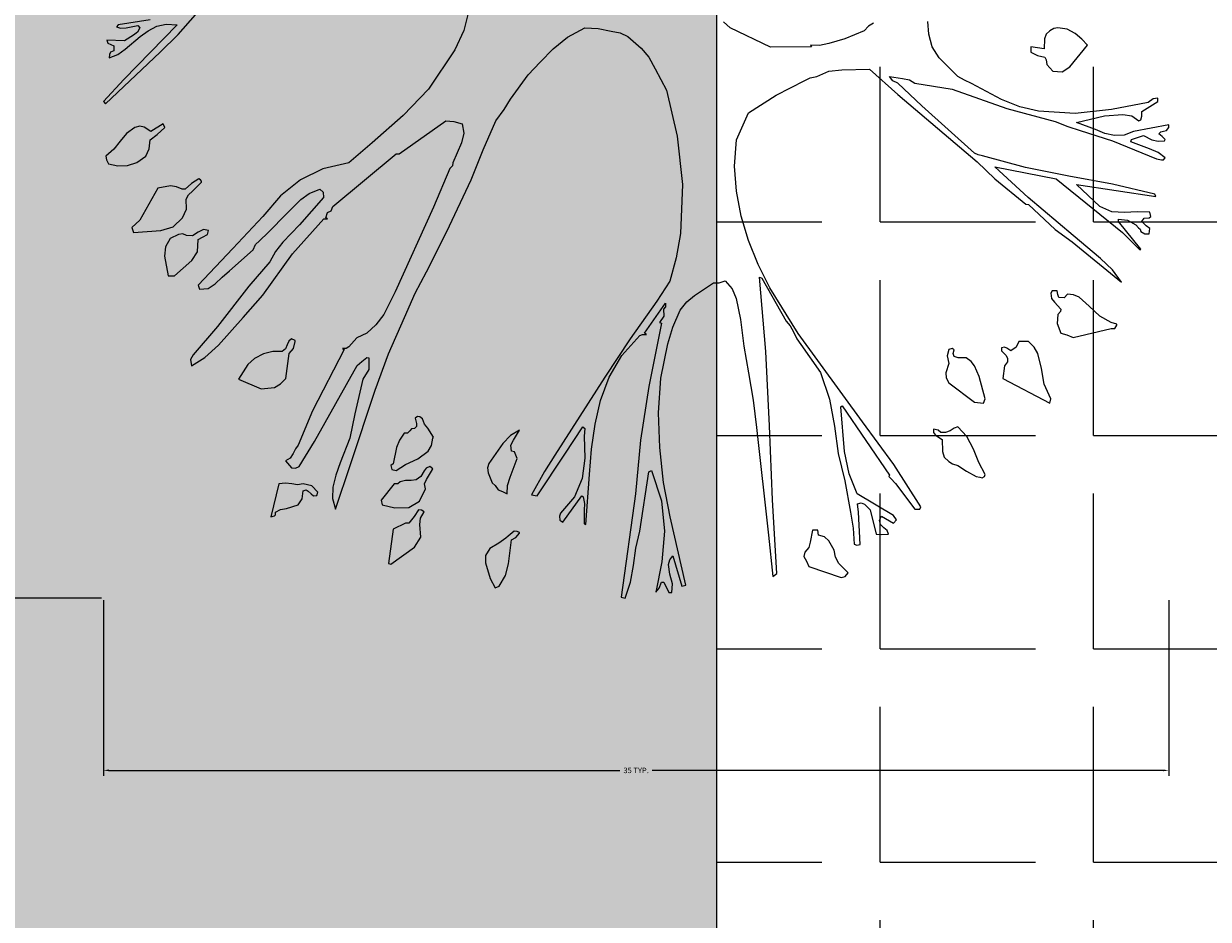
# Model space of a CAD drawing. Units: inches. Extents: x 84 to 1044, y -280 to 906.
# Tile 11 of 105: x 482 to 521, y -79 to -49. Entities that reach past the tile are written whole.
import ezdxf

# ---------------------------------------------------------------- set-up
doc = ezdxf.new("R2010")
doc.units = ezdxf.units.IN
for name, color, linetype, lineweight in [('A-ANNO-DIMS', 2, 'Continuous', 18), ('L-HRDS', 32, 'Continuous', 18), ('L-PLNT', 114, 'Continuous', 15)]:
    doc.layers.add(name, color=color, linetype=linetype, lineweight=lineweight)
doc.layers.add('L-HRDS-PATT', color=23, linetype='Continuous', lineweight=9, true_color=0xc2877b)
doc.layers.add('L-PLNT-PATT', color=9, linetype='Continuous', lineweight=9, true_color=0xafd9aa)
doc.styles.get("Standard").update_dxf_attribs({"font": 'arial.ttf'})
doc.dimstyles.get("Standard").update_dxf_attribs({"dimtxt": 0.18, "dimasz": 0.18, "dimexe": 0.18, "dimexo": 0.0625, "dimgap": 0.09, "dimtad": 0, "dimtih": 1, "dimtoh": 1, "dimdec": 4, "dimzin": 0, "dimdsep": 46, "dimtxsty": 'Standard', "dimcen": 0.09, "dimadec": 0, "dimazin": 0, "dimtfac": 1, "dimtdec": 4, "dimtofl": 0, "dimtmove": 0, "dimatfit": 3, "dimfxl": 1, "dimtolj": 1, "dimtzin": 0, "dimarcsym": 0})

# ---------------------------------------------------------------- blocks, each defined once
blk = doc.blocks.new('A$C37E508DF')
for p, q in [((0.9287, 0.7825), (0.936, 0.7542)), ((1.3151, 0.7487), (1.2919, 0.7752)), ((0.1244, 0.7504), (0.1351, 0.7559)), ((0.1351, 0.7559), (0.1471, 0.7577)), ((0.1471, 0.7577), (0.1527, 0.7568)), ((0.1527, 0.7568), (0.1578, 0.7538)), ((0.3186, 0.7491), (0.3199, 0.7662)), ((0.3919, 0.7641), (0.3988, 0.7598)), ((0.3988, 0.7598), (0.4043, 0.7538)), ((0.5287, 0.7319), (0.5823, 0.7577)), ((0.5823, 0.7577), (0.5913, 0.7658)), ((0.7577, 0.7568), (0.7401, 0.7534)), ((0.7752, 0.7577), (0.7577, 0.7568)), ((0.798, 0.7452), (0.7752, 0.7577)), ((1.3309, 0.7624), (1.3164, 0.7615)), ((1.3164, 0.7615), (1.3871, 0.6891)), ((1.3434, 0.7598), (1.3309, 0.7624)), ((1.355, 0.7538), (1.3434, 0.7598)), ((1.352, 0.7684), (1.3948, 0.7615)), ((1.3687, 0.7607), (1.3657, 0.7577)), ((1.3657, 0.7577), (1.3691, 0.7521)), ((1.3841, 0.7577), (1.3687, 0.7607)), ((1.3914, 0.7572), (1.3841, 0.7577)), ((1.397, 0.759), (1.3914, 0.7572)), ((1.3948, 0.7615), (1.397, 0.759)), ((0.1081, 0.7349), (0.1153, 0.7427)), ((0.1153, 0.7427), (0.1244, 0.7504)), ((0.1578, 0.7538), (0.1629, 0.7491)), ((0.1629, 0.7491), (0.1651, 0.7431)), ((0.1651, 0.7431), (0.1655, 0.7298)), ((0.3139, 0.7324), (0.3186, 0.7491)), ((0.4043, 0.7538), (0.4301, 0.7431)), ((0.4301, 0.7431), (0.4515, 0.7371)), ((0.7182, 0.7461), (0.7002, 0.7307)), ((0.7285, 0.7512), (0.7182, 0.7461)), ((0.7401, 0.7534), (0.7285, 0.7512)), ((0.8173, 0.7298), (0.798, 0.7452)), ((0.936, 0.7542), (0.9476, 0.7285)), ((1.3391, 0.7255), (1.3151, 0.7487)), ((1.3653, 0.7461), (1.355, 0.7538)), ((1.3854, 0.7294), (1.3653, 0.7461)), ((1.3691, 0.7521), (1.3743, 0.7482)), ((1.3743, 0.7482), (1.3863, 0.7405)), ((1.3863, 0.7405), (1.4099, 0.7414)), ((1.4099, 0.7414), (1.4086, 0.7375)), ((0.1312, 0.7058), (0.1081, 0.7349)), ((0.1655, 0.7298), (0.1831, 0.7324)), ((0.1831, 0.7255), (0.1741, 0.7208)), ((0.1831, 0.7324), (0.1831, 0.7255)), ((0.3049, 0.7178), (0.3139, 0.7324)), ((0.4515, 0.7371), (0.4635, 0.7341)), ((0.4635, 0.7341), (0.4755, 0.7349)), ((0.4755, 0.7349), (0.4742, 0.7324)), ((0.4742, 0.7324), (0.5287, 0.7319)), ((0.7002, 0.7307), (0.6903, 0.7186)), ((0.8344, 0.7122), (0.8173, 0.7298)), ((0.9476, 0.7285), (0.9828, 0.6762)), ((1.4116, 0.6569), (1.3391, 0.7255)), ((1.3953, 0.7221), (1.3854, 0.7294)), ((1.4086, 0.7375), (1.4004, 0.7337)), ((1.4004, 0.7337), (1.4004, 0.7272)), ((1.4004, 0.7272), (1.4047, 0.7255)), ((1.4047, 0.7255), (1.406, 0.7221)), ((0.1621, 0.7092), (0.1539, 0.7002)), ((0.1629, 0.7152), (0.1621, 0.7092)), ((0.1646, 0.7186), (0.1629, 0.7152)), ((0.1741, 0.7208), (0.1646, 0.7186)), ((0.28, 0.6933), (0.3049, 0.7178)), ((0.6903, 0.7186), (0.6818, 0.7032)), ((0.8503, 0.6951), (0.8344, 0.7122)), ((1.4064, 0.7178), (1.3953, 0.7221)), ((1.406, 0.7221), (1.4064, 0.7178)), ((0.1415, 0.6994), (0.1312, 0.7058)), ((0.1539, 0.7002), (0.1415, 0.6994)), ((0.271, 0.6882), (0.28, 0.6933)), ((0.3709, 0.6933), (0.3533, 0.6903)), ((0.3975, 0.7028), (0.3598, 0.6693)), ((0.3662, 0.6873), (0.3709, 0.6933)), ((0.4339, 0.7019), (0.3975, 0.7028)), ((0.4515, 0.7002), (0.4339, 0.7019)), ((0.4674, 0.6933), (0.4515, 0.7002)), ((0.476, 0.6912), (0.4674, 0.6933)), ((0.6818, 0.7032), (0.6667, 0.6749)), ((0.8739, 0.6629), (0.8503, 0.6951)), ((0.2877, 0.6762), (0.2152, 0.6505)), ((0.2221, 0.6625), (0.262, 0.6839)), ((0.262, 0.6839), (0.271, 0.6882)), ((0.337, 0.6843), (0.2877, 0.6762)), ((0.328, 0.6543), (0.3598, 0.6843)), ((0.3443, 0.6886), (0.337, 0.6843)), ((0.3533, 0.6903), (0.3443, 0.6886)), ((0.3598, 0.6843), (0.3662, 0.6873)), ((0.4832, 0.6878), (0.476, 0.6912)), ((0.521, 0.6685), (0.4832, 0.6878)), ((0.9828, 0.6762), (1.0162, 0.6415)), ((1.3871, 0.6891), (1.4141, 0.6599)), ((0.0146, 0.6599), (0.0146, 0.6642)), ((0.0146, 0.6642), (0.0206, 0.6633)), ((0.0206, 0.6633), (0.0274, 0.6586)), ((0.1977, 0.6526), (0.2221, 0.6625)), ((0.3598, 0.6693), (0.2543, 0.5797)), ((0.5578, 0.6449), (0.521, 0.6685)), ((0.6667, 0.6749), (0.6526, 0.614)), ((0.8824, 0.6492), (0.8739, 0.6629)), ((0.036, 0.6466), (0.0146, 0.6599)), ((0.0274, 0.6586), (0.0759, 0.6492)), ((0.0356, 0.6406), (0.036, 0.6466)), ((0.0759, 0.6492), (0.1244, 0.644)), ((0.1244, 0.644), (0.1728, 0.647)), ((0.2152, 0.6505), (0.1509, 0.6333)), ((0.1728, 0.647), (0.1977, 0.6526)), ((0.2581, 0.5913), (0.328, 0.6543)), ((0.5737, 0.6089), (0.5578, 0.6449)), ((0.8932, 0.6342), (0.8824, 0.6492)), ((1.4141, 0.6599), (1.4116, 0.6569)), ((0, 0.629), (0.0467, 0.62)), ((0, 0.6252), (0, 0.629)), ((0.0369, 0.6355), (0.0356, 0.6406)), ((0.0399, 0.6342), (0.0369, 0.6355)), ((0.0489, 0.641), (0.0399, 0.6342)), ((0.0609, 0.6428), (0.0489, 0.641)), ((0.0853, 0.641), (0.0609, 0.6428)), ((0.1226, 0.632), (0.0853, 0.641)), ((0.0973, 0.6226), (0.1226, 0.632)), ((0.1509, 0.6333), (0.1342, 0.6265)), ((0.9103, 0.5956), (0.8932, 0.6342)), ((0.9382, 0.6303), (0.936, 0.6179)), ((0.9493, 0.6333), (0.9382, 0.6303)), ((0.9596, 0.6342), (0.9493, 0.6333)), ((1.0218, 0.5904), (0.9596, 0.6342)), ((1.0162, 0.6415), (1.0574, 0.605)), ((1.3327, 0.6252), (1.3348, 0.6303)), ((1.3348, 0.6303), (1.3511, 0.62)), ((0.003, 0.6213), (0, 0.6252)), ((0.0069, 0.6204), (0.003, 0.6213)), ((0.0107, 0.6196), (0.0069, 0.6204)), ((0.0086, 0.6132), (0.0133, 0.617)), ((0.0133, 0.617), (0.0107, 0.6196)), ((0.0334, 0.6145), (0.0223, 0.6089)), ((0.0416, 0.6119), (0.0334, 0.6145)), ((0.0467, 0.62), (0.0592, 0.6153)), ((0.0592, 0.6153), (0.072, 0.6149)), ((0.072, 0.6149), (0.0849, 0.6175)), ((0.1175, 0.6213), (0.0746, 0.6076)), ((0.0849, 0.6175), (0.0973, 0.6226)), ((0.1342, 0.6265), (0.1175, 0.6213)), ((0.6526, 0.614), (0.6457, 0.5497)), ((0.936, 0.6179), (0.939, 0.605)), ((1.343, 0.6162), (1.3327, 0.6252)), ((1.352, 0.6089), (1.343, 0.6162)), ((1.3511, 0.62), (1.3601, 0.6256)), ((1.3601, 0.6256), (1.3661, 0.6269)), ((1.3661, 0.6269), (1.3725, 0.6252)), ((1.3725, 0.6252), (1.3837, 0.6175)), ((1.3837, 0.6175), (1.3918, 0.6072)), ((0.0047, 0.6093), (0.0086, 0.6132)), ((0.0056, 0.6076), (0.0047, 0.6093)), ((0.0141, 0.6072), (0.0056, 0.6076)), ((0.0223, 0.6089), (0.0141, 0.6072)), ((0.0746, 0.6076), (0.0163, 0.5836)), ((0.0257, 0.5969), (0.0506, 0.6063)), ((0.0493, 0.6093), (0.0416, 0.6119)), ((0.0506, 0.6063), (0.0493, 0.6093)), ((0.5763, 0.5741), (0.5737, 0.6089)), ((0.939, 0.605), (0.9506, 0.5784)), ((1.0574, 0.605), (1.0883, 0.5784)), ((1.3533, 0.5969), (1.352, 0.6089)), ((1.3918, 0.6072), (1.4004, 0.5964)), ((0.0047, 0.5849), (0.0141, 0.5921)), ((0.0069, 0.5823), (0.0047, 0.5849)), ((0.0099, 0.5823), (0.0069, 0.5823)), ((0.0163, 0.5836), (0.0099, 0.5823)), ((0.0141, 0.5921), (0.0257, 0.5969)), ((0.1904, 0.5724), (0.2474, 0.5879)), ((0.2474, 0.5879), (0.253, 0.5892)), ((0.253, 0.5892), (0.2581, 0.5913)), ((0.9262, 0.5557), (0.9103, 0.5956)), ((1.0256, 0.5904), (1.0218, 0.5904)), ((1.1097, 0.5205), (1.0256, 0.5904)), ((1.358, 0.5874), (1.3533, 0.5969)), ((1.37, 0.5789), (1.358, 0.5874)), ((1.4004, 0.5964), (1.4111, 0.5874)), ((1.4103, 0.5823), (1.4077, 0.5771)), ((1.4111, 0.5874), (1.4103, 0.5823)), ((0.1325, 0.5608), (0.1904, 0.5724)), ((0.2311, 0.5729), (0.1496, 0.557)), ((0.1869, 0.5325), (0.2311, 0.5729)), ((0.2543, 0.5797), (0.2311, 0.557)), ((0.5737, 0.5407), (0.5763, 0.5741)), ((0.9506, 0.5784), (0.951, 0.5746)), ((0.951, 0.5746), (0.9545, 0.5711)), ((0.9545, 0.5711), (0.9759, 0.5193)), ((1.0883, 0.5784), (1.123, 0.5703)), ((1.123, 0.5703), (1.1526, 0.5557)), ((1.3824, 0.575), (1.37, 0.5789)), ((1.3953, 0.5746), (1.3824, 0.575)), ((1.4077, 0.5771), (1.3953, 0.5746)), ((0.1496, 0.557), (0.0613, 0.4858)), ((0.0746, 0.5501), (0.1325, 0.5608)), ((0.2311, 0.557), (0.1899, 0.5235)), ((0.9583, 0.4871), (0.9262, 0.5557)), ((1.1526, 0.5557), (1.1792, 0.5347)), ((1.2842, 0.554), (1.2855, 0.5557)), ((1.2842, 0.5527), (1.2842, 0.554)), ((1.2958, 0.5407), (1.2842, 0.5527)), ((1.2855, 0.5557), (1.2876, 0.557)), ((1.2876, 0.557), (1.2971, 0.551)), ((1.2971, 0.551), (1.3057, 0.5433)), ((0.1226, 0.5497), (0.0171, 0.5338)), ((0.0171, 0.5338), (0.0184, 0.5368)), ((0.0184, 0.5368), (0.0746, 0.5501)), ((0.0917, 0.5205), (0.1226, 0.5497)), ((0.5677, 0.5077), (0.5737, 0.5407)), ((0.6457, 0.5497), (0.6483, 0.4845)), ((1.1226, 0.5394), (1.1221, 0.5325)), ((1.1268, 0.5433), (1.1226, 0.5394)), ((1.141, 0.5377), (1.1268, 0.5433)), ((1.1521, 0.5296), (1.141, 0.5377)), ((1.1792, 0.5347), (1.2027, 0.5072)), ((1.3014, 0.536), (1.2958, 0.5407)), ((1.3044, 0.53), (1.3014, 0.536)), ((1.3057, 0.5433), (1.3099, 0.5433)), ((1.3099, 0.5433), (1.3172, 0.5467)), ((1.3172, 0.5467), (1.3254, 0.548)), ((1.3254, 0.548), (1.3421, 0.5446)), ((1.3421, 0.5446), (1.3657, 0.5021)), ((0.0755, 0.5133), (0.0917, 0.5205)), ((0.1269, 0.482), (0.1869, 0.5325)), ((0.1861, 0.5231), (0.1509, 0.4897)), ((0.1899, 0.5235), (0.1861, 0.5231)), ((0.9759, 0.5193), (1.0269, 0.4069)), ((1.1118, 0.5145), (1.1097, 0.5205)), ((1.1221, 0.5325), (1.1539, 0.4961)), ((1.1706, 0.5111), (1.1521, 0.5296)), ((1.3039, 0.5167), (1.3044, 0.53)), ((0.024, 0.5072), (0.0253, 0.5128)), ((0.0262, 0.5055), (0.024, 0.5072)), ((0.0253, 0.5128), (0.042, 0.5133)), ((0.0326, 0.5047), (0.0262, 0.5055)), ((0.036, 0.5004), (0.0326, 0.5047)), ((0.042, 0.5133), (0.0587, 0.5124)), ((0.0669, 0.5034), (0.0549, 0.5021)), ((0.0587, 0.5124), (0.0755, 0.5133)), ((0.0669, 0.5004), (0.0669, 0.5034)), ((0.5578, 0.4751), (0.5677, 0.5077)), ((1.117, 0.5124), (1.1118, 0.5145)), ((1.1191, 0.5055), (1.117, 0.5124)), ((1.117, 0.5042), (1.1191, 0.5055)), ((1.1217, 0.5042), (1.117, 0.5042)), ((1.1633, 0.4575), (1.1217, 0.5042)), ((1.1955, 0.4858), (1.1706, 0.5111)), ((1.2027, 0.5072), (1.2426, 0.4644)), ((1.3091, 0.5055), (1.3039, 0.5167)), ((1.3215, 0.4935), (1.3091, 0.5055)), ((0.0253, 0.491), (0.03, 0.4948)), ((0.0262, 0.4841), (0.0253, 0.491)), ((0.03, 0.4948), (0.036, 0.5004)), ((0.0369, 0.4639), (0.0669, 0.5004)), ((0.0382, 0.4905), (0.0369, 0.4871)), ((0.0403, 0.4922), (0.0382, 0.4905)), ((0.0437, 0.4961), (0.0403, 0.4922)), ((0.0549, 0.5021), (0.0437, 0.4961)), ((0.1509, 0.4897), (0.1282, 0.4734)), ((1.1539, 0.4961), (1.1762, 0.4729)), ((1.2748, 0.4884), (1.2812, 0.4897)), ((1.2761, 0.4832), (1.2748, 0.4884)), ((1.2812, 0.4897), (1.2885, 0.4862)), ((1.3382, 0.4884), (1.3215, 0.4935)), ((1.3743, 0.4858), (1.3382, 0.4884)), ((1.3657, 0.5021), (1.3764, 0.4927)), ((1.3764, 0.4927), (1.3743, 0.4858)), ((0.0317, 0.4841), (0.0262, 0.4841)), ((0.0369, 0.4871), (0.0317, 0.4841)), ((0.0613, 0.4858), (0.0386, 0.4627)), ((0.1282, 0.4734), (0.0626, 0.4198)), ((0.0905, 0.4515), (0.1269, 0.482)), ((0.545, 0.4434), (0.5578, 0.4751)), ((0.6483, 0.4845), (0.6539, 0.4524)), ((0.9853, 0.4335), (0.9583, 0.4871)), ((1.1762, 0.4729), (1.1856, 0.4605)), ((1.207, 0.4747), (1.1955, 0.4858)), ((1.2122, 0.47), (1.207, 0.4747)), ((1.2825, 0.4798), (1.2761, 0.4832)), ((1.2885, 0.4764), (1.2825, 0.4798)), ((1.2885, 0.4862), (1.2962, 0.4815)), ((1.2894, 0.4601), (1.2885, 0.4764)), ((1.2962, 0.4815), (1.3039, 0.482)), ((1.3039, 0.482), (1.3087, 0.4841)), ((1.3087, 0.4841), (1.3147, 0.4832)), ((1.3147, 0.4832), (1.3258, 0.4777)), ((1.3258, 0.4777), (1.3318, 0.4669)), ((0.0386, 0.4627), (0.0369, 0.4639)), ((1.2027, 0.4026), (1.1633, 0.4575)), ((1.1856, 0.4605), (1.1933, 0.4468)), ((1.2156, 0.4627), (1.2122, 0.47)), ((1.2469, 0.4348), (1.2156, 0.4627)), ((1.2426, 0.4644), (1.2885, 0.4159)), ((1.2967, 0.4485), (1.2894, 0.4601)), ((1.3318, 0.4669), (1.3331, 0.4545)), ((0.0746, 0.4361), (0.0905, 0.4515)), ((0.5295, 0.4125), (0.545, 0.4434)), ((0.6539, 0.4524), (0.6625, 0.4211)), ((1.1933, 0.4468), (1.2212, 0.4146)), ((1.3082, 0.4386), (1.2967, 0.4485)), ((1.3331, 0.4545), (1.3284, 0.4284)), ((0.0626, 0.4198), (0.0746, 0.4361)), ((0.5403, 0.4254), (0.5081, 0.3679)), ((0.5347, 0.3276), (0.5433, 0.4266)), ((0.5433, 0.4266), (0.5403, 0.4254)), ((1.0003, 0.4052), (0.9853, 0.4335)), ((1.2568, 0.4266), (1.2469, 0.4348)), ((1.2658, 0.4176), (1.2568, 0.4266)), ((1.3198, 0.4284), (1.3082, 0.4386)), ((1.3284, 0.4284), (1.3198, 0.4284)), ((0.4922, 0.3516), (0.5295, 0.4125)), ((0.5797, 0.4112), (0.5741, 0.3983)), ((0.5887, 0.4215), (0.5797, 0.4112)), ((0.5969, 0.4189), (0.5887, 0.4215)), ((0.6046, 0.4189), (0.5969, 0.4189)), ((0.6295, 0.4022), (0.6046, 0.4189)), ((0.6625, 0.4211), (0.6796, 0.3945)), ((1.2212, 0.4146), (1.2628, 0.361)), ((1.2752, 0.4116), (1.2658, 0.4176)), ((1.2868, 0.4108), (1.2752, 0.4116)), ((1.2885, 0.4159), (1.2868, 0.4108)), ((0.1055, 0.388), (0.1192, 0.4001)), ((0.1192, 0.4001), (0.1265, 0.4031)), ((0.1265, 0.4031), (0.1346, 0.4039)), ((0.1346, 0.4039), (0.1389, 0.3992)), ((0.1389, 0.3992), (0.1458, 0.3996)), ((0.1518, 0.3932), (0.1432, 0.3842)), ((0.1458, 0.3996), (0.1471, 0.4035)), ((0.1471, 0.4035), (0.1484, 0.4082)), ((0.1484, 0.4082), (0.1548, 0.4082)), ((0.1556, 0.3983), (0.1518, 0.3932)), ((0.1548, 0.4082), (0.1565, 0.4052)), ((0.1565, 0.4052), (0.1556, 0.3983)), ((0.5741, 0.3983), (0.5686, 0.3705)), ((0.6397, 0.3936), (0.6295, 0.4022)), ((0.6487, 0.3825), (0.6397, 0.3936)), ((0.6796, 0.3945), (0.7148, 0.3447)), ((1.0145, 0.373), (1.0003, 0.4052)), ((1.0269, 0.4069), (1.0419, 0.3769)), ((1.2289, 0.373), (1.2027, 0.4026)), ((0.0917, 0.3748), (0.1055, 0.388)), ((0.1432, 0.3842), (0.1436, 0.3808)), ((0.1436, 0.3808), (0.1471, 0.3769)), ((0.6582, 0.3602), (0.6487, 0.3825)), ((0.6959, 0.352), (0.668, 0.3919)), ((0.668, 0.3919), (0.668, 0.3872)), ((0.668, 0.3872), (0.6706, 0.3842)), ((0.6706, 0.3842), (0.6702, 0.3748)), ((0.069, 0.364), (0.0763, 0.3662)), ((0.069, 0.3627), (0.069, 0.364)), ((0.0716, 0.3585), (0.069, 0.3627)), ((0.0763, 0.3662), (0.0917, 0.3748)), ((0.1484, 0.3649), (0.1432, 0.352)), ((0.1471, 0.3769), (0.1484, 0.3649)), ((0.5025, 0.3619), (0.4982, 0.3537)), ((0.5081, 0.3679), (0.5025, 0.3619)), ((0.5686, 0.3705), (0.5643, 0.3349)), ((0.6702, 0.3748), (0.6762, 0.3662)), ((0.6762, 0.3662), (0.6732, 0.3653)), ((0.6732, 0.3653), (0.6903, 0.2813)), ((1.0359, 0.3246), (1.0145, 0.373)), ((1.0419, 0.3769), (1.0527, 0.3632)), ((1.0527, 0.3632), (1.0647, 0.352)), ((1.2615, 0.3362), (1.2289, 0.373)), ((0.0763, 0.3585), (0.0716, 0.3585)), ((0.1269, 0.3464), (0.0763, 0.3585)), ((0.1355, 0.3499), (0.1269, 0.3464)), ((0.1432, 0.352), (0.1355, 0.3499)), ((0.4065, 0.2345), (0.4922, 0.3516)), ((0.4982, 0.3537), (0.4939, 0.3447)), ((0.665, 0.3379), (0.6582, 0.3602)), ((0.6933, 0.3503), (0.6959, 0.352)), ((0.6985, 0.3503), (0.6933, 0.3503)), ((0.7023, 0.349), (0.6985, 0.3503)), ((0.7259, 0.3224), (0.7023, 0.349)), ((1.0647, 0.352), (1.078, 0.346)), ((1.078, 0.346), (1.0883, 0.334)), ((1.2628, 0.361), (1.2949, 0.3233)), ((0.1737, 0.325), (0.1788, 0.3336)), ((0.1788, 0.3336), (0.1861, 0.3409)), ((0.1861, 0.3409), (0.199, 0.3409)), ((0.199, 0.3409), (0.2024, 0.3336)), ((0.2024, 0.3336), (0.2097, 0.3289)), ((0.2097, 0.3289), (0.2148, 0.3323)), ((0.2148, 0.3323), (0.2182, 0.3336)), ((0.2182, 0.3336), (0.2221, 0.3327)), ((0.2221, 0.3327), (0.2221, 0.3289)), ((0.2851, 0.3302), (0.2877, 0.3319)), ((0.2877, 0.3319), (0.292, 0.3306)), ((0.292, 0.3306), (0.2941, 0.322)), ((0.4884, 0.337), (0.4622, 0.2997)), ((0.4939, 0.3447), (0.4884, 0.337)), ((0.5643, 0.3349), (0.5578, 0.2993)), ((0.6745, 0.2924), (0.665, 0.3379)), ((0.7148, 0.3447), (0.7487, 0.2937)), ((1.0883, 0.334), (1.0921, 0.3319)), ((1.0921, 0.3319), (1.0968, 0.3319)), ((1.0968, 0.3319), (1.0947, 0.3306)), ((1.0947, 0.3306), (1.1367, 0.2491)), ((1.1599, 0.3426), (1.1646, 0.3447)), ((1.1599, 0.3413), (1.1599, 0.3426)), ((1.162, 0.3319), (1.1599, 0.3413)), ((1.1676, 0.325), (1.162, 0.3319)), ((1.1646, 0.3447), (1.168, 0.3417)), ((1.168, 0.3417), (1.1702, 0.3366)), ((1.1702, 0.3366), (1.1727, 0.3314)), ((1.1727, 0.3314), (1.177, 0.3276)), ((1.2795, 0.3199), (1.2615, 0.3362)), ((0.1689, 0.3053), (0.1737, 0.325)), ((0.2161, 0.3224), (0.214, 0.3186)), ((0.214, 0.3186), (0.214, 0.3139)), ((0.2221, 0.3289), (0.2161, 0.3224)), ((0.2577, 0.3087), (0.2624, 0.3147)), ((0.2624, 0.3147), (0.2689, 0.3194)), ((0.2689, 0.3194), (0.2796, 0.3194)), ((0.2796, 0.3194), (0.2847, 0.3211)), ((0.2847, 0.3211), (0.2864, 0.325)), ((0.2864, 0.325), (0.2851, 0.3302)), ((0.2941, 0.322), (0.292, 0.3117)), ((0.53, 0.229), (0.5347, 0.3276)), ((0.7427, 0.2937), (0.7259, 0.3224)), ((1.0535, 0.2766), (1.0359, 0.3246)), ((1.0647, 0.3199), (1.0617, 0.3194)), ((1.0617, 0.3194), (1.0617, 0.304)), ((1.0711, 0.3147), (1.0647, 0.3199)), ((1.0775, 0.3092), (1.0711, 0.3147)), ((1.1719, 0.292), (1.1676, 0.325)), ((1.177, 0.3276), (1.1895, 0.3276)), ((1.1895, 0.3276), (1.2019, 0.3246)), ((1.2019, 0.3246), (1.2135, 0.3186)), ((1.2135, 0.3186), (1.2225, 0.3104)), ((1.2975, 0.3087), (1.2795, 0.3199)), ((1.2949, 0.3233), (1.2988, 0.3173)), ((1.2988, 0.3173), (1.2975, 0.3087)), ((0.1655, 0.2843), (0.1689, 0.3053)), ((0.214, 0.3139), (0.2182, 0.3087)), ((0.2182, 0.3087), (0.2204, 0.292)), ((0.2517, 0.2946), (0.2577, 0.3087)), ((0.292, 0.3117), (0.2959, 0.2993)), ((0.2959, 0.2993), (0.2954, 0.2928)), ((0.4622, 0.2997), (0.4502, 0.2645)), ((0.5578, 0.2993), (0.5518, 0.2633)), ((1.0617, 0.304), (1.0698, 0.2911)), ((1.1341, 0.2084), (1.0775, 0.3092)), ((1.2225, 0.3104), (1.2349, 0.2911)), ((0.1565, 0.265), (0.1655, 0.2843)), ((0.2204, 0.292), (0.1578, 0.259)), ((0.2436, 0.265), (0.2517, 0.2946)), ((0.292, 0.286), (0.2581, 0.2607)), ((0.2954, 0.2928), (0.292, 0.286)), ((0.6775, 0.2465), (0.6745, 0.2924)), ((0.7542, 0.2628), (0.7427, 0.2937)), ((0.7487, 0.2937), (0.8151, 0.1899)), ((1.0698, 0.2911), (1.0805, 0.2448)), ((1.1792, 0.2847), (1.1719, 0.292)), ((1.1873, 0.28), (1.1792, 0.2847)), ((1.2349, 0.2911), (1.2049, 0.2783)), ((0.6903, 0.2813), (0.7015, 0.2101)), ((1.0861, 0.1775), (1.0535, 0.2766)), ((1.2049, 0.2783), (1.1873, 0.28)), ((0.1578, 0.259), (0.1565, 0.265)), ((0.2461, 0.259), (0.2436, 0.265)), ((0.2581, 0.2607), (0.2461, 0.259)), ((0.4335, 0.2556), (0.3709, 0.1634)), ((0.4305, 0.1951), (0.4352, 0.2543)), ((0.4352, 0.2543), (0.4335, 0.2556)), ((0.4502, 0.2645), (0.4438, 0.2285)), ((0.5518, 0.2633), (0.5475, 0.2268)), ((0.7615, 0.2311), (0.7542, 0.2628)), ((0.6758, 0.2002), (0.6775, 0.2465)), ((0.9879, 0.2311), (0.9905, 0.2384)), ((0.9905, 0.2384), (0.9943, 0.241)), ((0.9943, 0.241), (0.9973, 0.2414)), ((0.9973, 0.2414), (1.0003, 0.2393)), ((1.0003, 0.2393), (0.9986, 0.232)), ((1.0805, 0.2448), (1.087, 0.2127)), ((1.1367, 0.2491), (1.1556, 0.2032)), ((0.268, 0.2148), (0.28, 0.2277)), ((0.28, 0.2277), (0.2851, 0.226)), ((0.2851, 0.226), (0.2903, 0.2225)), ((0.2903, 0.2225), (0.2963, 0.22)), ((0.2963, 0.22), (0.3027, 0.2204)), ((0.3027, 0.2204), (0.3061, 0.2234)), ((0.3061, 0.2234), (0.3122, 0.2247)), ((0.3122, 0.2247), (0.3122, 0.22)), ((0.3649, 0.1775), (0.4065, 0.2345)), ((0.4438, 0.2285), (0.4391, 0.1921)), ((0.5261, 0.1308), (0.53, 0.229)), ((0.5475, 0.2268), (0.5313, 0.084)), ((0.7662, 0.1981), (0.7615, 0.2311)), ((0.7778, 0.2277), (0.7752, 0.2255)), ((0.7752, 0.2255), (0.7761, 0.2152)), ((0.8018, 0.1912), (0.7778, 0.2277)), ((0.8619, 0.2234), (0.8739, 0.2161)), ((0.87, 0.2101), (0.8619, 0.2234)), ((0.9759, 0.214), (0.9836, 0.226)), ((0.9836, 0.226), (0.9879, 0.2311)), ((0.9986, 0.232), (0.9986, 0.2281)), ((0.9986, 0.2281), (1.0012, 0.2255)), ((1.0012, 0.2255), (1.0051, 0.2251)), ((1.0051, 0.2251), (1.0076, 0.2225)), ((1.0076, 0.2225), (1.0106, 0.2195)), ((0.2594, 0.1981), (0.268, 0.2148)), ((0.301, 0.211), (0.3002, 0.1951)), ((0.3096, 0.2165), (0.301, 0.211)), ((0.3122, 0.22), (0.3096, 0.2165)), ((0.7015, 0.2101), (0.7079, 0.1389)), ((0.7761, 0.2152), (0.7752, 0.1861)), ((0.8734, 0.2032), (0.87, 0.2101)), ((0.8739, 0.2161), (0.8841, 0.2054)), ((0.8841, 0.2054), (0.9026, 0.1792)), ((0.9768, 0.2127), (0.9759, 0.214)), ((0.9789, 0.2028), (0.9768, 0.2127)), ((1.0106, 0.2195), (1.0149, 0.2191)), ((1.0149, 0.2191), (1.0214, 0.2101)), ((1.0214, 0.2101), (1.0252, 0.2002)), ((1.087, 0.2127), (1.0998, 0.1797)), ((1.1543, 0.1749), (1.1341, 0.2084)), ((0.2521, 0.1805), (0.2594, 0.1981)), ((0.3002, 0.1951), (0.298, 0.1874)), ((0.4241, 0.1651), (0.4305, 0.1951)), ((0.4391, 0.1921), (0.4301, 0.1561)), ((0.6706, 0.1539), (0.6758, 0.2002)), ((0.7688, 0.1646), (0.7662, 0.1981)), ((0.8383, 0.1359), (0.8018, 0.1912)), ((0.8151, 0.1899), (0.8288, 0.1685)), ((0.8649, 0.1857), (0.8687, 0.1947)), ((0.8687, 0.1947), (0.8726, 0.1955)), ((0.8726, 0.1955), (0.8734, 0.2032)), ((0.9832, 0.1955), (0.9789, 0.2028)), ((0.9969, 0.1852), (0.9832, 0.1955)), ((1.0252, 0.2002), (1.0295, 0.1788)), ((1.1556, 0.2032), (1.1594, 0.1985)), ((1.1594, 0.1985), (1.1624, 0.1921)), ((1.1624, 0.1921), (1.1663, 0.1861)), ((0.2436, 0.1642), (0.2521, 0.1805)), ((0.28, 0.1762), (0.2684, 0.1689)), ((0.2873, 0.1788), (0.28, 0.1762)), ((0.292, 0.1818), (0.2873, 0.1788)), ((0.298, 0.1874), (0.292, 0.1818)), ((0.3293, 0.1213), (0.3649, 0.1775)), ((0.7752, 0.1861), (0.7787, 0.1591)), ((0.8743, 0.1608), (0.8649, 0.1857)), ((0.9026, 0.1792), (0.9043, 0.1732)), ((0.9043, 0.1732), (0.9035, 0.1668)), ((0.9768, 0.1719), (0.9811, 0.1749)), ((0.9811, 0.1749), (0.9858, 0.1728)), ((1.0132, 0.1779), (0.9969, 0.1852)), ((1.0256, 0.1698), (1.0132, 0.1779)), ((1.0295, 0.1788), (1.0325, 0.1762)), ((1.0325, 0.1762), (1.0312, 0.1711)), ((1.1063, 0.1183), (1.0861, 0.1775)), ((1.0998, 0.1797), (1.1058, 0.1634)), ((1.1594, 0.1728), (1.1543, 0.1749)), ((1.1646, 0.1732), (1.1594, 0.1728)), ((1.1727, 0.1827), (1.1646, 0.1732)), ((1.1663, 0.1861), (1.1727, 0.1827)), ((0.2448, 0.1616), (0.2436, 0.1642)), ((0.2478, 0.1599), (0.2448, 0.1616)), ((0.2508, 0.1608), (0.2478, 0.1599)), ((0.2556, 0.1616), (0.2508, 0.1608)), ((0.2684, 0.1689), (0.2556, 0.1616)), ((0.3692, 0.1591), (0.3628, 0.1526)), ((0.3718, 0.1616), (0.3692, 0.1591)), ((0.3709, 0.1634), (0.3718, 0.1616)), ((0.4138, 0.1389), (0.4241, 0.1651)), ((0.6865, 0.1698), (0.6732, 0.1295)), ((0.6903, 0.1681), (0.6865, 0.1698)), ((0.7023, 0.0892), (0.6903, 0.1681)), ((0.774, 0.0982), (0.7688, 0.1646)), ((0.7787, 0.1591), (0.789, 0.1346)), ((0.8288, 0.1685), (0.846, 0.1376)), ((0.8777, 0.1496), (0.8743, 0.1608)), ((0.9035, 0.1668), (0.8983, 0.1535)), ((0.9776, 0.1711), (0.9768, 0.1719)), ((0.9853, 0.1578), (0.9776, 0.1711)), ((0.9879, 0.1518), (0.9853, 0.1578)), ((0.9858, 0.1728), (0.9884, 0.1694)), ((0.9884, 0.1694), (0.9931, 0.1616)), ((0.9931, 0.1616), (0.9991, 0.1574)), ((0.9991, 0.1574), (1.0059, 0.1565)), ((1.0312, 0.1711), (1.0256, 0.1698)), ((1.1058, 0.1634), (1.1097, 0.1475)), ((0.3628, 0.1526), (0.337, 0.1183)), ((0.4301, 0.1561), (0.4224, 0.1145)), ((0.662, 0.108), (0.6706, 0.1539)), ((0.8781, 0.1389), (0.8777, 0.1496)), ((0.8846, 0.1419), (0.8781, 0.1389)), ((0.8902, 0.1441), (0.8846, 0.1419)), ((0.894, 0.1496), (0.8902, 0.1441)), ((0.8983, 0.1535), (0.894, 0.1496)), ((0.9866, 0.1453), (0.9879, 0.1518)), ((0.9948, 0.1291), (0.9866, 0.1453)), ((1.0059, 0.1565), (1.0132, 0.1565)), ((1.0132, 0.1565), (1.0205, 0.1548)), ((1.0205, 0.1548), (1.0235, 0.1522)), ((1.0235, 0.1522), (1.0282, 0.1518)), ((1.0282, 0.1518), (1.0454, 0.1303)), ((1.1097, 0.1475), (1.1101, 0.1325)), ((1.1298, 0.1411), (1.1376, 0.1492)), ((1.1376, 0.1492), (1.1491, 0.1518)), ((1.1423, 0.1423), (1.1384, 0.1389)), ((1.1449, 0.1441), (1.1423, 0.1423)), ((1.1491, 0.1428), (1.1449, 0.1441)), ((1.1491, 0.1518), (1.1564, 0.1505)), ((1.1504, 0.132), (1.1491, 0.1428)), ((1.1564, 0.1505), (1.1642, 0.1518)), ((1.1642, 0.1518), (1.1727, 0.1531)), ((1.1727, 0.1531), (1.1813, 0.1518)), ((1.1813, 0.1518), (1.192, 0.108)), ((0.3653, 0.1098), (0.4138, 0.1389)), ((0.4082, 0.1269), (0.4039, 0.1248)), ((0.4134, 0.1256), (0.4082, 0.1269)), ((0.5205, 0.033), (0.5261, 0.1308)), ((0.6732, 0.1295), (0.6693, 0.0892)), ((0.7079, 0.1389), (0.7268, 0.0013)), ((0.7774, 0.1346), (0.7757, 0.1261)), ((0.7757, 0.1261), (0.7761, 0.117)), ((0.7791, 0.1359), (0.7774, 0.1346)), ((0.8044, 0.1012), (0.7791, 0.1359)), ((0.789, 0.1346), (0.8074, 0.1132)), ((0.846, 0.1376), (0.8383, 0.1359)), ((1.0089, 0.1205), (0.9948, 0.1291)), ((1.0454, 0.1303), (1.0441, 0.1239)), ((1.1101, 0.1325), (1.1063, 0.1183)), ((1.1311, 0.1364), (1.1298, 0.1411)), ((1.1354, 0.1359), (1.1311, 0.1364)), ((1.1384, 0.1389), (1.1354, 0.1359)), ((1.1556, 0.1239), (1.1504, 0.132)), ((0.3306, 0.1183), (0.3293, 0.1213)), ((0.337, 0.1183), (0.3306, 0.1183)), ((0.3962, 0.1175), (0.3885, 0.0853)), ((0.4039, 0.1248), (0.3962, 0.1175)), ((0.4099, 0.0716), (0.4121, 0.1145)), ((0.4121, 0.1145), (0.4134, 0.1256)), ((0.4224, 0.1145), (0.4189, 0.093)), ((0.7761, 0.117), (0.7761, 0.099)), ((0.8074, 0.1132), (0.8087, 0.1089)), ((0.9884, 0.1149), (0.9918, 0.117)), ((0.9935, 0.1063), (0.9884, 0.1149)), ((0.9918, 0.117), (0.9961, 0.1175)), ((0.9961, 0.1175), (1.0016, 0.1085)), ((1.0274, 0.12), (1.0089, 0.1205)), ((1.0441, 0.1239), (1.0274, 0.12)), ((1.1714, 0.1192), (1.1556, 0.1239)), ((1.1792, 0.1179), (1.1714, 0.1192)), ((1.186, 0.1145), (1.1792, 0.1179)), ((1.1856, 0.111), (1.186, 0.1145)), ((1.1873, 0.1093), (1.1856, 0.111)), ((0.3615, 0.1042), (0.3653, 0.1098)), ((0.3653, 0.0999), (0.3615, 0.1042)), ((0.3812, 0.1089), (0.3653, 0.0999)), ((0.3782, 0.0935), (0.3825, 0.0978)), ((0.3842, 0.1037), (0.3812, 0.1089)), ((0.3825, 0.0978), (0.3842, 0.1037)), ((0.641, 0.0172), (0.662, 0.108)), ((0.7761, 0.099), (0.774, 0.0982)), ((0.8083, 0.1037), (0.8044, 0.1012)), ((0.8087, 0.1089), (0.8083, 0.1037)), ((0.9931, 0.081), (0.9943, 0.0982)), ((0.9943, 0.0982), (0.9935, 0.1063)), ((1.0016, 0.1085), (1.0089, 0.0999)), ((1.0089, 0.0999), (1.0132, 0.0999)), ((1.0132, 0.0999), (1.0295, 0.0917)), ((1.192, 0.108), (1.1873, 0.1093)), ((0.3722, 0.0853), (0.3739, 0.09)), ((0.3808, 0.0845), (0.3722, 0.0853)), ((0.3739, 0.09), (0.3782, 0.0935)), ((0.3885, 0.0853), (0.3808, 0.0845)), ((0.4189, 0.093), (0.4176, 0.072)), ((0.4515, 0.0763), (0.4571, 0.0815)), ((0.4571, 0.0815), (0.4648, 0.084)), ((0.4648, 0.084), (0.4657, 0.0905)), ((0.4657, 0.0905), (0.473, 0.0905)), ((0.473, 0.0905), (0.476, 0.0746)), ((0.5313, 0.084), (0.5257, 0.0291)), ((0.6693, 0.0892), (0.6728, 0.0484)), ((0.7075, 0.0665), (0.7023, 0.0892)), ((0.8619, 0.0875), (0.8649, 0.0887)), ((0.8619, 0.0866), (0.8619, 0.0875)), ((0.8666, 0.0806), (0.8619, 0.0866)), ((0.8649, 0.0887), (0.8691, 0.0892)), ((0.8726, 0.0776), (0.8666, 0.0806)), ((0.8691, 0.0892), (0.8769, 0.0827)), ((0.8769, 0.0827), (0.8799, 0.0797)), ((0.8799, 0.0797), (0.8893, 0.0733)), ((1.0012, 0.0677), (0.9931, 0.081)), ((1.0295, 0.0917), (1.0359, 0.0463)), ((0.4142, 0.0707), (0.4099, 0.0716)), ((0.4176, 0.072), (0.4142, 0.0707)), ((0.4425, 0.0544), (0.4442, 0.0639)), ((0.4442, 0.0639), (0.4515, 0.0763)), ((0.476, 0.0746), (0.4777, 0.0673)), ((0.4777, 0.0673), (0.4832, 0.0613)), ((0.7105, 0.0437), (0.7075, 0.0665)), ((0.8764, 0.0459), (0.8726, 0.0776)), ((0.8893, 0.0733), (0.9013, 0.066)), ((0.9013, 0.066), (0.9069, 0.057)), ((1.0325, 0.0454), (1.0012, 0.0677)), ((0.4378, 0.0463), (0.4425, 0.0544)), ((0.4811, 0.0493), (0.4777, 0.0424)), ((0.4845, 0.0553), (0.4811, 0.0493)), ((0.4832, 0.0613), (0.4845, 0.0553)), ((0.6582, 0.0562), (0.6466, 0.0159)), ((0.6625, 0.051), (0.6582, 0.0562)), ((0.6642, 0.045), (0.6625, 0.051)), ((0.6728, 0.0484), (0.6809, 0.0082)), ((0.9069, 0.057), (0.9069, 0.0471)), ((0.4258, 0.0339), (0.4378, 0.0463)), ((0.4296, 0.0291), (0.4258, 0.0339)), ((0.4777, 0.0424), (0.4348, 0.0274)), ((0.5257, 0.0291), (0.5205, 0.033)), ((0.659, 0.0193), (0.6625, 0.0321)), ((0.6625, 0.0321), (0.6642, 0.045)), ((0.7144, 0.0214), (0.7105, 0.0437)), ((0.8807, 0.0304), (0.8764, 0.0459)), ((0.9069, 0.0471), (0.9009, 0.0261)), ((1.0359, 0.0463), (1.0325, 0.0454)), ((0.4348, 0.0274), (0.4296, 0.0291)), ((0.6466, 0.0159), (0.641, 0.0172)), ((0.6595, 0.0077), (0.659, 0.0193)), ((0.6702, 0.0214), (0.6637, 0.0077)), ((0.6732, 0.0214), (0.6702, 0.0214)), ((0.6766, 0.0133), (0.6732, 0.0214)), ((0.7216, 0), (0.7144, 0.0214)), ((0.8889, 0.0159), (0.8807, 0.0304)), ((0.894, 0.0137), (0.8889, 0.0159)), ((0.9009, 0.0261), (0.894, 0.0137)), ((0.6637, 0.0077), (0.6595, 0.0077)), ((0.6809, 0.0082), (0.6766, 0.0133)), ((0.7268, 0.0013), (0.7216, 0))]:
    blk.add_line(p, q)
blk = doc.blocks.new('*D28')
at = {"layer": 'A-ANNO-DIMS', "color": 0, "lineweight": -2, "transparency": 16777216}
for p, q in [((484.443, -30.627), (478.69, -30.627)), ((478.87, -30.807), (478.87, -49.227)), ((478.87, -68.013), (478.87, -49.593)), ((484.443, -68.193), (478.69, -68.193))]:
    blk.add_line(p, q, dxfattribs=at)
at = {"layer": 'A-ANNO-DIMS', "color": 0, "transparency": 16777216}
for points in [[(478.84, -30.807), (478.9, -30.807), (478.87, -30.627)], [(478.84, -68.013), (478.9, -68.013), (478.87, -68.193)]]:
    blk.add_solid(points, dxfattribs=at)
at = {"layer": 'Defpoints', "color": 0, "transparency": 16777216}
for p in [(478.87, -30.627), (484.505, -30.627), (484.505, -68.193)]:
    blk.add_point(p, dxfattribs=at)
at = {"layer": 'A-ANNO-DIMS', "color": 0, "transparency": 16777216, "insert": (478.87, -49.41), "char_height": 0.18, "attachment_point": 5}
blk.add_mtext('\\A1;SHRUB 38 TYP.', dxfattribs=at)
blk = doc.blocks.new('*D29')
at = {"layer": 'A-ANNO-DIMS', "color": 0, "lineweight": -2, "transparency": 16777216}
for p, q in [((484.505, -68.255), (484.505, -74.007)), ((519.355, -68.255), (519.355, -74.007)), ((484.685, -73.827), (501.402, -73.827)), ((519.175, -73.827), (502.458, -73.827))]:
    blk.add_line(p, q, dxfattribs=at)
at = {"layer": 'A-ANNO-DIMS', "color": 0, "transparency": 16777216}
for points in [[(484.685, -73.797), (484.685, -73.857), (484.505, -73.827)], [(519.175, -73.797), (519.175, -73.857), (519.355, -73.827)]]:
    blk.add_solid(points, dxfattribs=at)
at = {"layer": 'Defpoints', "color": 0, "transparency": 16777216}
for p in [(484.505, -68.193), (519.355, -68.193), (484.505, -73.827)]:
    blk.add_point(p, dxfattribs=at)
at = {"layer": 'A-ANNO-DIMS', "color": 0, "transparency": 16777216, "insert": (501.93, -73.827), "char_height": 0.18, "attachment_point": 5}
blk.add_mtext('\\A1;35 TYP.', dxfattribs=at)

msp = doc.modelspace()

# ---------------------------------------------------------------- hatches: boundary and pattern name
at = {"layer": 'L-HRDS-PATT', "transparency": 33554567}
h = msp.add_hatch(dxfattribs=at)
h.set_pattern_fill('ANGLE', color=256)
h.set_pattern_definition([(0, (0, 0), (0, 6.985), [5.08, -1.905]), (90, (0, 0), (-6.985, 4e-16), [5.08, -1.905])])
h.paths.add_polyline_path([(650.074, 31.12), (504.574, 31.12), (504.574, -112.88), (504.574, -121.88), (624.574, -121.88), (624.574, -112.88), (650.074, -112.88)])
at = {"layer": 'L-PLNT-PATT', "transparency": 33554597}
h = msp.add_hatch(color=256, dxfattribs=at)
h.dxf.hatch_style = 1
h.paths.add_polyline_path([(504.574, -40.88), (455.074, -40.88), (455.074, -112.88), (504.574, -112.88)])

# ---------------------------------------------------------------- linework, layer by layer
at = {"layer": 'L-HRDS'}
msp.add_line((504.574, -112.88), (504.574, 31.12), dxfattribs=at)

# ---------------------------------------------------------------- block references
at = {"layer": 'L-PLNT', "xscale": -24.64361536662419, "yscale": 24.64361536662419, "zscale": 24.64361536662419}
msp.add_blockref('A$C37E508DF', (519.355, -68.193), dxfattribs=at)

# ---------------------------------------------------------------- dimensions: what is measured, and where the dimension line sits
at = {"layer": 'A-ANNO-DIMS'}
for base, p1, p2, angle, text, picture, middle in [((478.87, -30.627), (484.505, -68.193), (484.505, -30.627), 90, 'SHRUB <> TYP.', '*D28', (478.87, -49.41)), ((484.505, -73.827), (519.355, -68.193), (484.505, -68.193), 180, '<> TYP.', '*D29', (501.93, -73.827))]:
    dim = msp.add_linear_dim(base=base, p1=p1, p2=p2, angle=angle, text=text, dimstyle='Standard', override={"dimdec": 0, "dimlfac": 1, "dimrnd": 0, "dimzin": 0, "dimdsep": 46, "dimlunit": 2}, dxfattribs=at)
    dim.commit()
    dim.dimension.update_dxf_attribs({"geometry": picture, "text_midpoint": middle})

doc.saveas('drawing.dxf')
